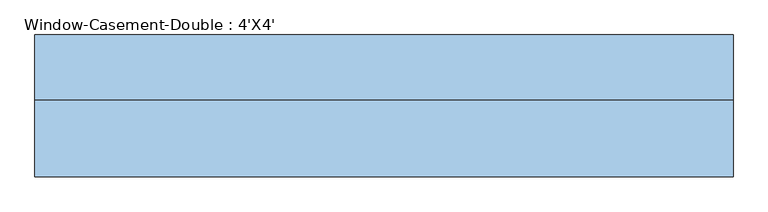
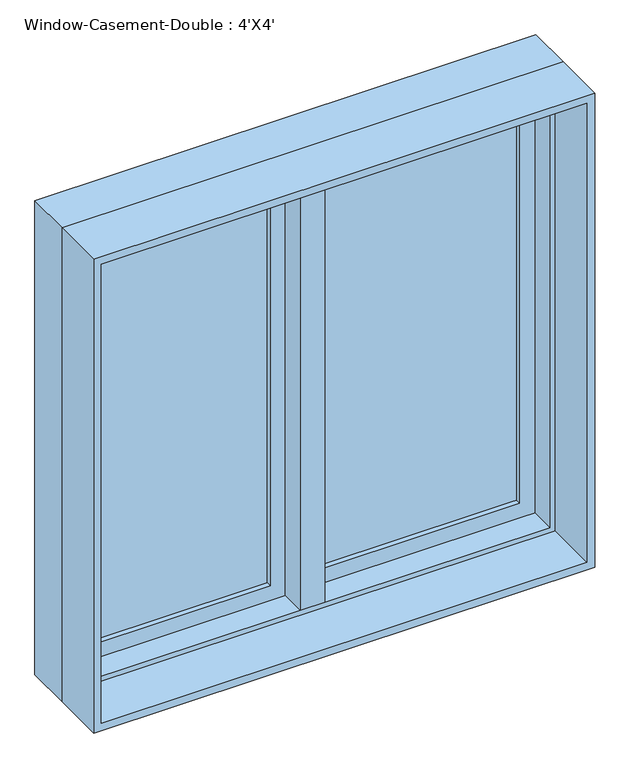
"""IFC4 building model written with IfcOpenShell, lengths in millimetres: window geometry, Window-Casement-Double : 4'X4'."""

from ifc_helpers import new_model, si_unit, frame, origin, place, context, project, spatial, polyline, outline, extrude, faceted_brep, source, transform, mapped, element, save


def window_casement_double_4_x4_af3140d2(model_context):
    return source(origin(), model_context, "Body", "SolidModel", [
        faceted_brep([(9.525, 133.35, 2120.9), (-9.525, 133.35, 2120.9), (-9.525, 82.55, 2120.9), (9.525, 82.55, 2120.9), (9.525, 133.35, 927.1), (9.525, 82.55, 927.1), (-9.525, 82.55, 927.1), (-9.525, 133.35, 927.1), (-9.525, 82.55, 946.15), (-9.525, 82.55, 2101.85), (-30.1625, 82.55, 946.15), (-30.1625, 82.55, 2101.85), (-30.1625, 19.05, 946.15), (-30.1625, 19.05, 2101.85), (30.1625, 19.05, 946.15), (30.1625, 19.05, 2101.85), (30.1625, 82.55, 946.15), (30.1625, 82.55, 2101.85), (9.525, 82.55, 946.15), (9.525, 82.55, 2101.85)], [[[0, 1, 2, 3]], [[4, 5, 6, 7]], [[1, 0, 4, 7]], [[2, 1, 7, 6, 8, 9]], [[9, 8, 10, 11]], [[11, 10, 12, 13]], [[13, 12, 14, 15]], [[15, 14, 16, 17]], [[17, 16, 18, 19]], [[0, 3, 19, 18, 5, 4]], [[18, 8, 6, 5]], [[9, 19, 3, 2]], [[8, 18, 16, 14, 12, 10]], [[19, 9, 11, 13, 15, 17]]]),
        extrude(outline(polyline([(-66.675, 114.3), (-66.675, 107.95), (-539.75, 107.95), (-539.75, 114.3), (-66.675, 114.3)])), frame((0.0, 0.0, 984.25), z_axis=(0.0, 0.0, 1.0), x_axis=(1.0, 0.0, 0.0)), (0.0, 0.0, 1.0), 1079.5),
        extrude(outline(polyline([(-539.75, 95.25), (-539.75, 101.6), (-66.675, 101.6), (-66.675, 95.25), (-539.75, 95.25)])), frame((0.0, 0.0, 984.25), z_axis=(0.0, 0.0, 1.0), x_axis=(1.0, 0.0, 0.0)), (0.0, 0.0, 1.0), 1079.5),
        extrude(outline(polyline([(539.75, 114.3), (539.75, 107.95), (66.675, 107.95), (66.675, 114.3), (539.75, 114.3)])), frame((0.0, 0.0, 984.25), z_axis=(0.0, 0.0, 1.0), x_axis=(1.0, 0.0, 0.0)), (0.0, 0.0, 1.0), 1079.5),
        extrude(outline(polyline([(66.675, 95.25), (66.675, 101.6), (539.75, 101.6), (539.75, 95.25), (66.675, 95.25)])), frame((0.0, 0.0, 984.25), z_axis=(0.0, 0.0, 1.0), x_axis=(1.0, 0.0, 0.0)), (0.0, 0.0, 1.0), 1079.5),
        extrude(outline(polyline([(2120.9, -596.9), (927.1, -596.9), (927.1, -9.525), (2120.9, -9.525), (2120.9, -596.9)]), holes=[polyline([(2063.75, -66.675), (984.25, -66.675), (984.25, -539.75), (2063.75, -539.75), (2063.75, -66.675)])]), frame((0.0, 82.55, 0.0), z_axis=(0.0, 1.0, 0.0), x_axis=(0.0, 0.0, 1.0)), (0.0, 0.0, 1.0), 44.45),
        extrude(outline(polyline([(927.1, 596.9), (2120.9, 596.9), (2120.9, 9.525), (927.1, 9.525), (927.1, 596.9)]), holes=[polyline([(984.25, 66.675), (2063.75, 66.675), (2063.75, 539.75), (984.25, 539.75), (984.25, 66.675)])]), frame((0.0, 82.55, 0.0), z_axis=(0.0, 1.0, 0.0), x_axis=(0.0, 0.0, 1.0)), (0.0, 0.0, 1.0), 44.45),
        extrude(outline(polyline([(2133.6, -609.6), (914.4, -609.6), (914.4, 609.6), (2133.6, 609.6), (2133.6, -609.6)]), holes=[polyline([(2114.55, 590.55), (933.45, 590.55), (933.45, -590.55), (2114.55, -590.55), (2114.55, 590.55)])]), frame((0.0, -114.3, 0.0), z_axis=(0.0, 1.0, 0.0), x_axis=(0.0, 0.0, 1.0)), (0.0, 0.0, 1.0), 133.35),
        faceted_brep([(577.85, 82.55, 2101.85), (577.85, 19.05, 2101.85), (-577.85, 19.05, 2101.85), (-577.85, 82.55, 2101.85), (596.9, 133.35, 2120.9), (596.9, 82.55, 2120.9), (-596.9, 82.55, 2120.9), (-596.9, 133.35, 2120.9), (609.6, 19.05, 2133.6), (609.6, 133.35, 2133.6), (-609.6, 133.35, 2133.6), (-609.6, 19.05, 2133.6), (-577.85, 19.05, 946.15), (-577.85, 82.55, 946.15), (-596.9, 82.55, 927.1), (-596.9, 133.35, 927.1), (-609.6, 133.35, 914.4), (-609.6, 19.05, 914.4), (577.85, 19.05, 946.15), (577.85, 82.55, 946.15), (596.9, 82.55, 927.1), (596.9, 133.35, 927.1), (609.6, 133.35, 914.4), (609.6, 19.05, 914.4)], [[[0, 1, 2, 3]], [[4, 5, 6, 7]], [[8, 9, 10, 11]], [[3, 2, 12, 13]], [[7, 6, 14, 15]], [[11, 10, 16, 17]], [[13, 12, 18, 19]], [[15, 14, 20, 21]], [[17, 16, 22, 23]], [[11, 17, 23, 8], [1, 18, 12, 2]], [[19, 18, 1, 0]], [[5, 20, 14, 6], [3, 13, 19, 0]], [[21, 20, 5, 4]], [[23, 22, 9, 8]], [[9, 22, 16, 10], [7, 15, 21, 4]]]),
    ])


if __name__ == "__main__":
    model = new_model("IFC4")
    model_context = context("Model", 3, world=origin())
    ifc_project = project(units=[si_unit("LENGTHUNIT", "METRE", prefix="MILLI")], contexts=[model_context])
    site = spatial("IfcSite", under=ifc_project)
    building = spatial("IfcBuilding", under=site)
    placement = place(None, origin())
    window_casement_double_4_x4_shape = window_casement_double_4_x4_af3140d2(model_context)
    element("IfcWindow", 1, ObjectType="Window-Casement-Double : 4'X4'", at=placement, inside=building, context=model_context, shape_type="MappedRepresentation", body=[
        mapped(window_casement_double_4_x4_shape, transform((0.0, 0.0, 0.0), x_axis=(1.0, 0.0, 0.0), y_axis=(0.0, 1.0, 0.0), z_axis=(0.0, 0.0, 1.0))),
    ])
    save(model, "model.ifc")

# Revit data of these elements
# Type "Window-Casement-Double : 4'X4'"
#   Type Mark = "30"
#   Fire Rating = "0.5h"
#   Assembly Code = "B2020100"
#   Analytic Construction = "Double glazing - domestic"
#   Frame Extension [instance default] = 0' - 0 1/4"
#   Window Inset [instance default] = 0' - 0"
#   Wall Thickness [instance default] = 0' - 6"
#   Interior Wall Closure [instance default] = 0' - 2 1/4"
#   Half Width = 2' - 0"
#   Visual Light Transmittance = 0.81
#   Thermal Resistance (R) = 1.8146 (h·ft²·°F)/BTU
#   Solar Heat Gain Coefficient = 0.76
#   Rough Width = 4' - 0 1/2"
#   Rough Height = 4' - 0 1/2"
#   Height = 4' - 0"
#   Heat Transfer Coefficient (U) = 0.5511 BTU/(h·ft²·°F)
#   Exterior Wall Closure [instance default] = 0' - 1 1/4"
#   Extension Jamb [instance default] = 0' - 2 1/4"
#   Default Sill Height = 3' - 0"
#   Width = 4' - 0"
#   Muntin Visibility = yes
#   Interior Trim Visibility [instance default] = yes
#   Exterior Trim Visibility [instance default] = yes
#   Extension Jamb Visibility [instance default] = yes
#   Interior Trim Material = Wood - Stained
#   Muntin Pattern = Muntin Pattern_2x2 : Muntin Pattern_2x2
#   Interior Trim = Trim-Window-Interior-Flat : Picture Frame
#   Interior Frame Material = Wood - Stained
#   Glass Panel Material = Glass
#   Exterior Trim Material = Clad - White
#   Exterior Trim = Trim-Window-Exterior-Flat : with Sill
#   Exterior Frame Material = Clad - White
#   Wall Closure = (empty or 0)
# Element 1 (IfcWindow, "Window-Casement-Double : 4'X4'")
#   Wall Thickness = 0' - 9"
#   Extension Jamb = 0' - 5 1/4"
#   Materials on its faces: "Wood - Stained", "Glass", "Clad - White"
# Materials
#   "Wood - Stained": class "Wood", colour RGB 224 178 126, transparency 0, Cost = 0
#   "Glass": class "Glass", colour RGB 0 128 192, transparency 0.75, Description = "Soda Lime Glass", Cost = 0
#   "Clad - White": class "Wood", colour RGB 242 242 238, transparency 0, Cost = 0
